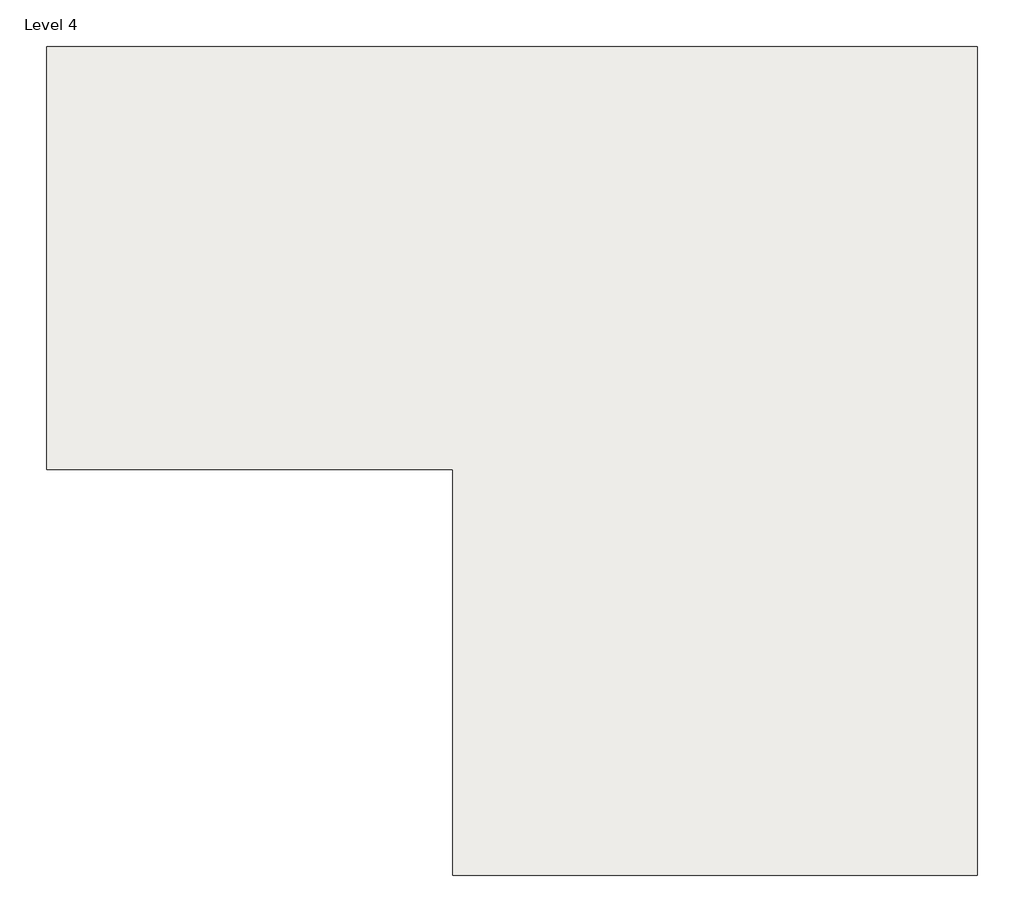
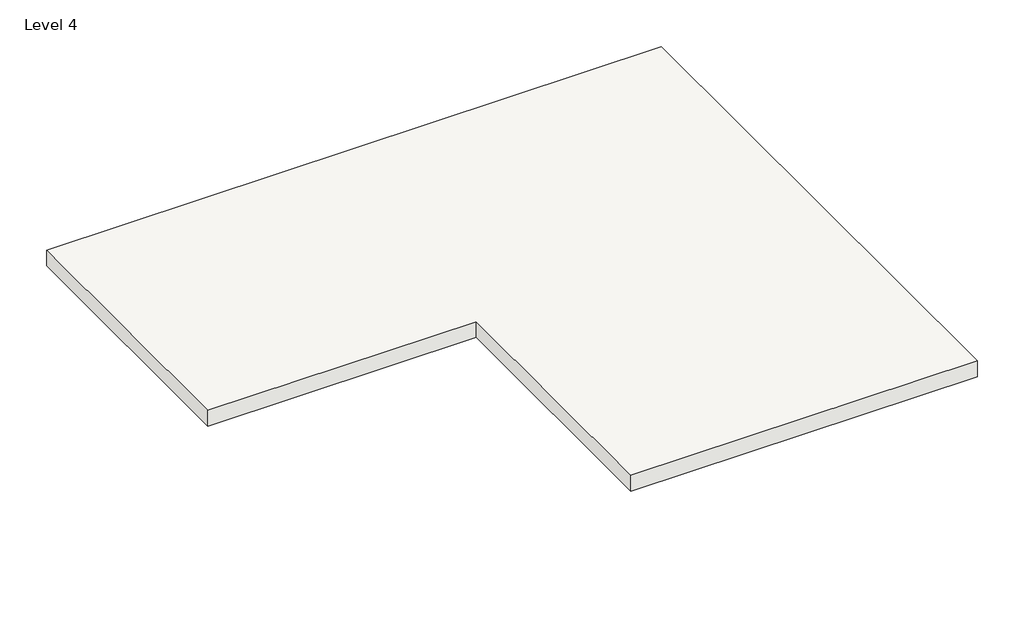
# One storey: 1 roof.
"""IFC4 building model written with IfcOpenShell, lengths in millimetres."""

from ifc_helpers import new_model, si_unit, frame, origin, place, context, project, spatial, polyline, outline, extrude, element, save

model = new_model("IFC4")

# Units and contexts
model_context = context("Model", 3, world=origin())
ifc_project = project(units=[si_unit("LENGTHUNIT", "METRE", prefix="MILLI")], contexts=[model_context])

# Site, building, storey
site = spatial("IfcSite", under=ifc_project)
building = spatial("IfcBuilding", under=site)
storey = spatial("IfcBuildingStorey", under=building, Name="Level 4", Elevation=10972.8)

# Roof
placement = place(None, origin())
element("IfcRoof", 1, ObjectType="Generic - 12\"", at=placement, inside=storey, context=model_context, shape_type="SweptSolid", body=[
    extrude(outline(polyline([(-12556.4681702, 9304.2612165), (-1380.4681702, 9304.2612165), (-1380.4681702, -652.5387835), (-7679.6681702, -652.5387835), (-7679.6681702, 4224.2612165), (-12556.4681702, 4224.2612165), (-12556.4681702, 9304.2612165)])), frame((0.0, 0.0, 10972.8), z_axis=(0.0, 0.0, 1.0), x_axis=(1.0, 0.0, 0.0)), (0.0, 0.0, 1.0), 304.8),
])

save(model, "model.ifc")

# Revit data of these elements
# Type "Generic - 12\""
#   Assembly Code = "B1020"
#   Layers, outside or top first: 1' - 0" no material (function 1)
# Element 1 (IfcRoof, "Generic - 12\"")
#   built-in parameter 1001705 = 37 (stored number, unit not read)
#   built-in parameter 1001710 = 33615
#   Phase Created = New Construction
#   Materials on its faces: "Default Roof"
# Materials
#   "Default Roof": colour RGB 88 101 114, transparency 0
